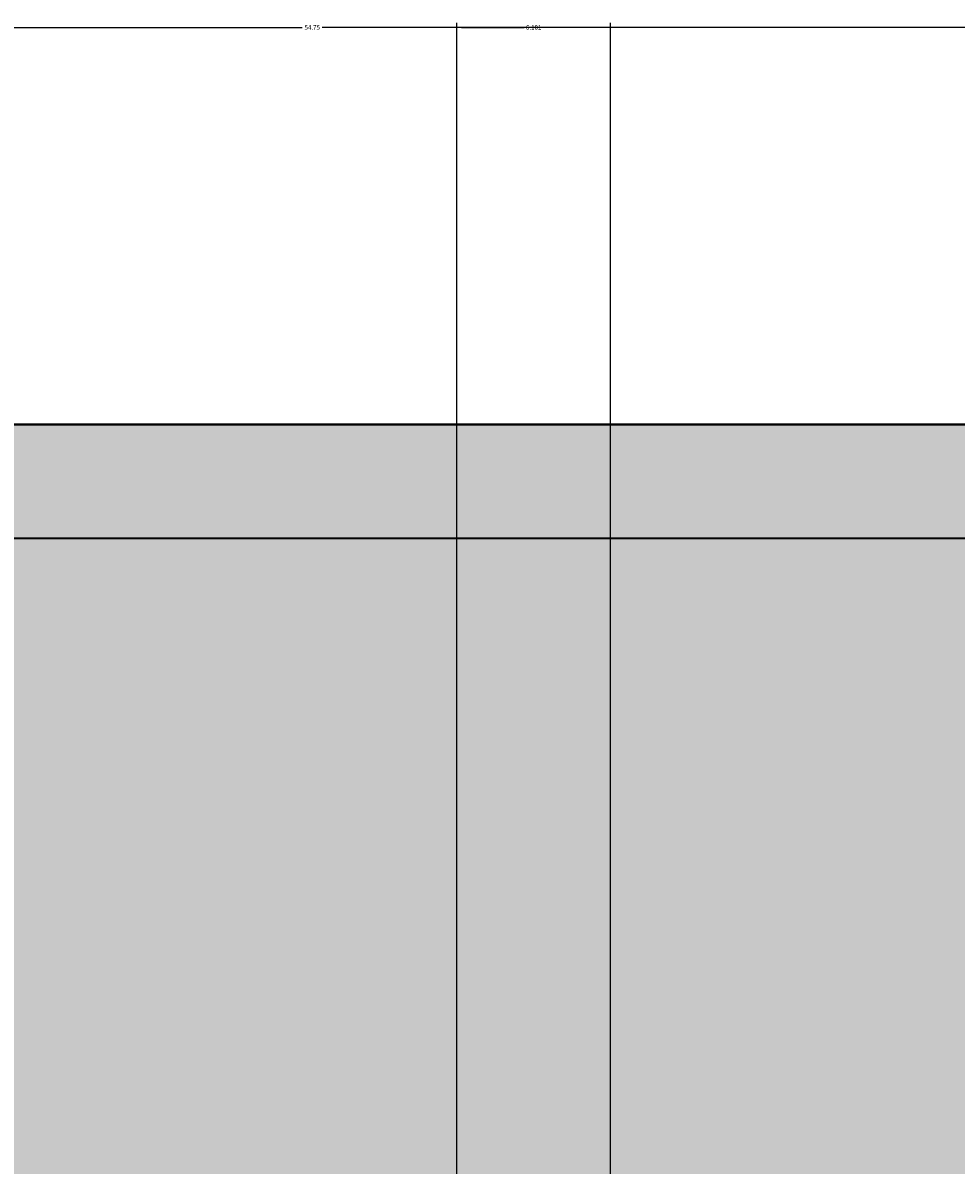
# Model space of a CAD drawing. Units: feet. Extents: x 2695 to 2912, y 795 to 1139.
# Tile 51 of 83: x 2732 to 2769, y 1093 to 1139. Entities that reach past the tile are written whole.
import ezdxf

# ---------------------------------------------------------------- set-up
doc = ezdxf.new("R2010")
doc.units = ezdxf.units.FT
for name, color, linetype, lineweight in [('A-ANNO-DIMS', 2, 'Continuous', 18), ('A-ELEV', 7, 'Continuous', 35), ('A-ELEV-PATT', 252, 'Continuous', 13)]:
    doc.layers.add(name, color=color, linetype=linetype, lineweight=lineweight)
doc.styles.get("Standard").update_dxf_attribs({"font": 'arial.ttf'})
doc.dimstyles.get("Standard").update_dxf_attribs({"dimtxt": 0.18, "dimasz": 0.18, "dimexe": 0.18, "dimexo": 0.0625, "dimgap": 0.09, "dimtad": 0, "dimtih": 1, "dimtoh": 1, "dimdec": 1, "dimzin": 0, "dimdsep": 46, "dimlunit": 3, "dimtxsty": 'Standard', "dimcen": 0.09, "dimadec": 0, "dimazin": 0, "dimtfac": 1, "dimtdec": 1, "dimtofl": 0, "dimtmove": 0, "dimatfit": 3, "dimfxl": 1, "dimtolj": 1, "dimtzin": 0, "dimarcsym": 0})

# ---------------------------------------------------------------- blocks, each defined once
blk = doc.blocks.new('*D8')
at = {"layer": 'A-ANNO-DIMS', "color": 0, "lineweight": -2, "transparency": 16777216}
for p, q in [((2715.885, 1050.373), (2715.885, 1138.886)), ((2770.636, 1122.993), (2770.636, 1138.886)), ((2716.065, 1138.706), (2742.866, 1138.706)), ((2770.456, 1138.706), (2743.655, 1138.706))]:
    blk.add_line(p, q, dxfattribs=at)
at = {"layer": 'A-ANNO-DIMS', "color": 0, "transparency": 16777216}
for points in [[(2716.065, 1138.736), (2716.065, 1138.676), (2715.885, 1138.706)], [(2770.456, 1138.736), (2770.456, 1138.676), (2770.636, 1138.706)]]:
    blk.add_solid(points, dxfattribs=at)
at = {"layer": 'Defpoints', "color": 0, "transparency": 16777216}
for p in [(2770.636, 1138.706), (2770.636, 1122.931), (2715.885, 1050.311)]:
    blk.add_point(p, dxfattribs=at)
at = {"layer": 'A-ANNO-DIMS', "color": 0, "transparency": 16777216, "insert": (2743.261, 1138.706), "char_height": 0.18, "attachment_point": 5}
blk.add_mtext('\\A1;54.75', dxfattribs=at)
blk = doc.blocks.new('*D26')
at = {"layer": 'A-ANNO-DIMS', "color": 0, "lineweight": -2, "transparency": 16777216}
for p, q in [((2749.011, 1048.168), (2749.011, 1138.886)), ((2755.112, 1048.168), (2755.112, 1138.886)), ((2749.191, 1138.706), (2751.685, 1138.706)), ((2754.932, 1138.706), (2752.439, 1138.706))]:
    blk.add_line(p, q, dxfattribs=at)
at = {"layer": 'A-ANNO-DIMS', "color": 0, "transparency": 16777216}
for points in [[(2749.191, 1138.736), (2749.191, 1138.676), (2749.011, 1138.706)], [(2754.932, 1138.736), (2754.932, 1138.676), (2755.112, 1138.706)]]:
    blk.add_solid(points, dxfattribs=at)
at = {"layer": 'Defpoints', "color": 0, "transparency": 16777216}
for p in [(2755.112, 1138.706), (2749.011, 1048.105), (2755.112, 1048.105)]:
    blk.add_point(p, dxfattribs=at)
at = {"layer": 'A-ANNO-DIMS', "color": 0, "transparency": 16777216, "insert": (2752.062, 1138.706), "char_height": 0.18, "attachment_point": 5}
blk.add_mtext('\\A1;6.101', dxfattribs=at)

msp = doc.modelspace()

# ---------------------------------------------------------------- hatches: boundary and pattern name
at = {"layer": 'A-ELEV-PATT'}
h = msp.add_hatch(color=256, dxfattribs=at)
h.set_gradient(color1=(255, 255, 255), tint=1)
h.paths.add_polyline_path([(2770.6361, 1122.9306), (2710.6361, 1122.9306), (2710.6361, 1118.4096), (2770.6361, 1118.4096)])
h.paths.add_polyline_path([(2890.6361, 1107.8588), (2770.6361, 1107.8588), (2770.6361, 1103.3378), (2890.6361, 1103.3378)])
h.paths.add_polyline_path([(2890.6361, 1062.9306), (2710.6361, 1062.9306), (2710.6361, 1056.9306), (2710.6361, 936.9306), (2710.6361, 924.3105), (2716.5358, 924.3105), (2890.6361, 924.3105), (2890.6361, 936.9306), (2715.8852, 936.9306), (2715.8852, 1050.3105), (2890.6361, 1050.3105)])
h.paths.add_polyline_path([(2716.5358, 924.3105), (2710.6361, 924.3105), (2710.6361, 810.9306), (2716.5358, 810.9306)])
h = msp.add_hatch(color=256, dxfattribs=at)
h.set_gradient(color1=(147, 149, 152), color2=(147, 149, 152), tint=1)
h.paths.add_polyline_path([(2770.6361, 1118.4096), (2710.6361, 1118.4096), (2710.6361, 1062.9306), (2770.6361, 1062.9306)])
h.paths.add_polyline_path([(2890.6361, 1103.3378), (2770.6361, 1103.3378), (2770.6361, 1062.9306), (2890.6361, 1062.9306)])
h.paths.add_polyline_path([(2730.7081, 1048.1052), (2755.1125, 1048.1052), (2755.1125, 936.9306), (2770.6361, 936.9306), (2770.6361, 1050.3105), (2715.8852, 1050.3105), (2715.8852, 936.9306), (2730.7081, 936.9306)])
h.paths.add_polyline_path([(2890.6361, 1050.3105), (2770.6361, 1050.3105), (2770.6361, 971.9673), (2778.0341, 971.9673), (2778.0341, 1020.8235), (2843.575, 1020.8235), (2843.575, 971.9673), (2890.6361, 971.9673)])
h.paths.add_polyline_path([(2888.1882, 970.7156), (2843.575, 970.7156), (2843.575, 964.8267), (2888.1882, 964.8267)])
h.paths.add_polyline_path([(2888.1882, 964.1328), (2843.575, 964.1328), (2843.575, 956.614), (2888.1882, 956.614)])
h.paths.add_polyline_path([(2888.1882, 955.9202), (2843.575, 955.9202), (2843.575, 949.2892), (2888.1882, 949.2892)])
h.paths.add_polyline_path([(2888.1882, 948.5954), (2843.575, 948.5954), (2843.575, 941.3507), (2888.1882, 941.3507)])
h.paths.add_polyline_path([(2888.1882, 940.6569), (2843.575, 940.6569), (2843.575, 936.9306), (2888.1882, 936.9306)])
h.paths.add_polyline_path([(2890.6361, 970.7156), (2888.9368, 970.7156), (2888.9368, 964.8267), (2890.6361, 964.8267)])
h.paths.add_polyline_path([(2890.6361, 964.1328), (2888.9368, 964.1328), (2888.9368, 956.614), (2890.6361, 956.614)])
h.paths.add_polyline_path([(2890.6361, 955.9202), (2888.9368, 955.9202), (2888.9368, 949.2892), (2890.6361, 949.2892)])
h.paths.add_polyline_path([(2890.6361, 940.6569), (2888.9368, 940.6569), (2888.9368, 936.9306), (2890.6361, 936.9306)])
h.paths.add_polyline_path([(2890.6361, 948.5954), (2888.9368, 948.5954), (2888.9368, 941.3507), (2890.6361, 941.3507)])
h.paths.add_polyline_path([(2772.5216, 970.7156), (2770.6361, 970.7156), (2770.6361, 964.8267), (2772.5216, 964.8267)])
h.paths.add_polyline_path([(2772.5216, 964.1328), (2770.6361, 964.1328), (2770.6361, 956.614), (2772.5216, 956.614)])
h.paths.add_polyline_path([(2772.5216, 955.9202), (2770.6361, 955.9202), (2770.6361, 949.2892), (2772.5216, 949.2892)])
h.paths.add_polyline_path([(2772.5216, 948.5954), (2770.6361, 948.5954), (2770.6361, 941.3507), (2772.5216, 941.3507)])
h.paths.add_polyline_path([(2772.5216, 940.6569), (2770.6361, 940.6569), (2770.6361, 936.9306), (2772.5216, 936.9306)])
h.paths.add_polyline_path([(2778.0341, 940.6569), (2773.2702, 940.6569), (2773.2702, 936.9306), (2778.0341, 936.9306)])
h.paths.add_polyline_path([(2778.0341, 970.7156), (2773.2702, 970.7156), (2773.2702, 964.8267), (2778.0341, 964.8267)])
h.paths.add_polyline_path([(2778.0341, 964.1328), (2773.2702, 964.1328), (2773.2702, 956.614), (2778.0341, 956.614)])
h.paths.add_polyline_path([(2778.0341, 955.9202), (2773.2702, 955.9202), (2773.2702, 949.2892), (2778.0341, 949.2892)])
h.paths.add_polyline_path([(2778.0341, 948.5954), (2773.2702, 948.5954), (2773.2702, 941.3507), (2778.0341, 941.3507)])
h.paths.add_polyline_path([(2810.0407, 940.6569), (2780.0341, 940.6569), (2780.0341, 936.9306), (2810.0407, 936.9306)])
h.paths.add_polyline_path([(2890.6361, 924.3105), (2770.6361, 924.3105), (2770.6361, 810.9306), (2773.5029, 810.9306), (2773.5029, 905.5143), (2805.9398, 905.5143), (2838.3767, 905.5143), (2838.3767, 810.9306), (2890.6361, 810.9306)])

# ---------------------------------------------------------------- linework, layer by layer
at = {"layer": 'A-ELEV'}
for p, q in [((2710.6361, 1122.9306), (2770.6361, 1122.9306)), ((2770.6361, 1122.9306), (2710.6361, 1122.9306)), ((2710.6361, 1118.4096), (2770.6361, 1118.4096))]:
    msp.add_line(p, q, dxfattribs=at)
msp.add_lwpolyline([(2710.6361, 1118.4096), (2770.6361, 1118.4096)], dxfattribs=at)

# ---------------------------------------------------------------- dimensions: what is measured, and where the dimension line sits
at = {"layer": 'A-ANNO-DIMS'}
for base, p1, p2, override, picture, middle in [((2770.6361, 1138.7056), (2715.8852, 1050.3105), (2770.6361, 1122.9306), {"dimdec": 2, "dimlfac": 1, "dimrnd": 0, "dimzin": 0, "dimdsep": 46, "dimlunit": 2}, '*D8', (2743.2606, 1138.7056)), ((2755.1125, 1138.7056), (2749.0114, 1048.1052), (2755.1125, 1048.1052), {"dimdec": 3, "dimlfac": 1, "dimrnd": 0, "dimzin": 0, "dimdsep": 46, "dimlunit": 2}, '*D26', (2752.0619, 1138.7056))]:
    dim = msp.add_linear_dim(base=base, p1=p1, p2=p2, dimstyle='Standard', override=override, dxfattribs=at)
    dim.commit()
    dim.dimension.update_dxf_attribs({"geometry": picture, "text_midpoint": middle})

doc.saveas('drawing.dxf')
